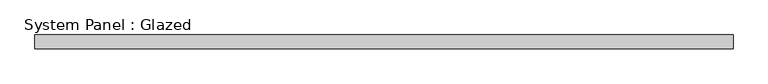
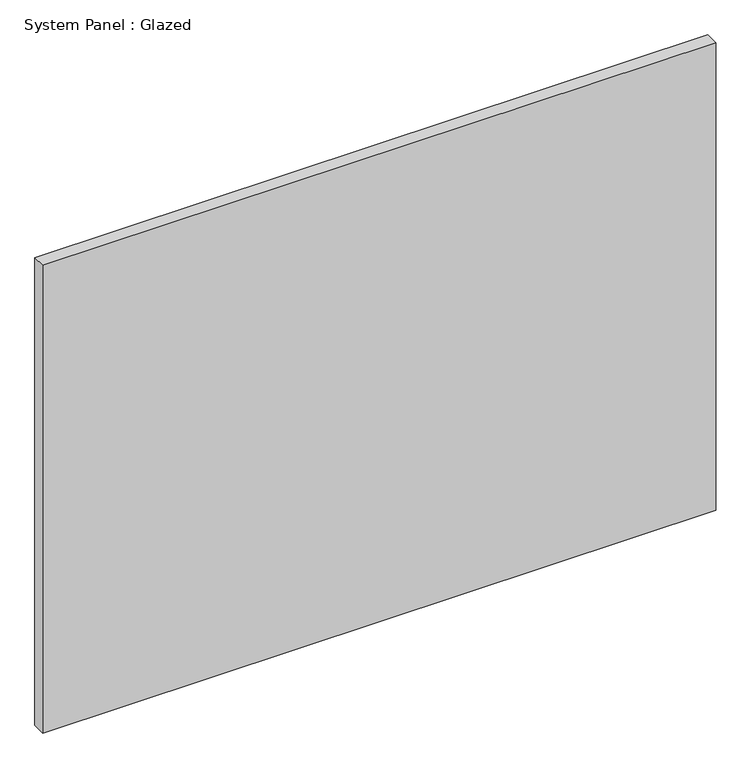
"""IFC4 building model written with IfcOpenShell, lengths in millimetres: plate geometry, System Panel : Glazed."""

from ifc_helpers import new_model, si_unit, origin, origin_with_axes, place, context, project, spatial, polyline, outline, extrude, source, transform, mapped, element, save


def system_panel_glazed_a94942f9(model_context):
    return source(origin(), model_context, "Body", "SweptSolid", [
        extrude(outline(polyline([(638.1750001, 19.05), (-638.1750001, 19.05), (-638.1750001, 44.45), (638.1750001, 44.45), (638.1750001, 19.05)])), origin_with_axes(), (0.0, 0.0, 1.0), 937.6833333),
    ])


if __name__ == "__main__":
    model = new_model("IFC4")
    model_context = context("Model", 3, world=origin())
    ifc_project = project(units=[si_unit("LENGTHUNIT", "METRE", prefix="MILLI")], contexts=[model_context])
    site = spatial("IfcSite", under=ifc_project)
    building = spatial("IfcBuilding", under=site)
    placement = place(None, origin())
    system_panel_glazed_shape = system_panel_glazed_a94942f9(model_context)
    element("IfcPlate", 1, ObjectType="System Panel : Glazed", at=placement, inside=building, context=model_context, shape_type="MappedRepresentation", body=[
        mapped(system_panel_glazed_shape, transform((0.0, 0.0, 0.0), x_axis=(1.0, 0.0, 0.0), y_axis=(0.0, 1.0, 0.0), z_axis=(0.0, 0.0, 1.0))),
    ])
    save(model, "model.ifc")

# Revit data of these elements
# Type "System Panel : Glazed"
#   Construction Type Id = "GSP4R"
#   Analytic Construction = "1/8 in Pilkington single glazing"
#   Visual Light Transmittance = 0.9
#   Solar Heat Gain Coefficient = 0.86
#   Heat Transfer Coefficient (U) = 1.18115 BTU/(h·ft²·°F)
#   Define Thermal Properties by = 1
# Element 1 (IfcPlate, "System Panel : Glazed")
#   Materials on its faces: "glass panel 223"
# Materials
#   "glass panel 223": class "Generic", colour RGB 120 120 120, transparency 0, Cost = 0
